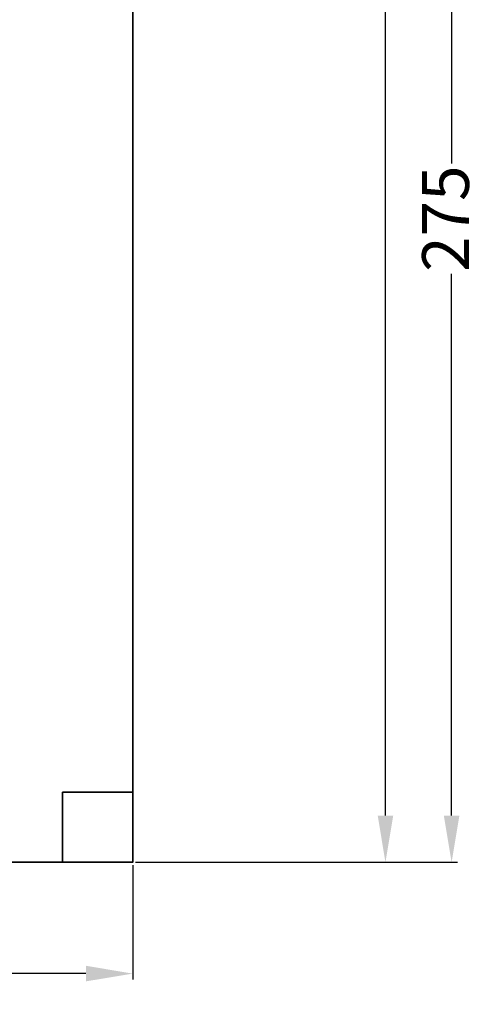
# Model space of a CAD drawing. Units: centimetres. Extents: x 2401 to 3632, y 2122 to 3526.
# Tile 4 of 10: x 3221 to 3320, y 2381 to 2591. Entities that reach past the tile are written whole.
import ezdxf

# ---------------------------------------------------------------- set-up
doc = ezdxf.new("R2010")
doc.units = ezdxf.units.CM
for name, color, linetype, lineweight in [('A-ANNO-DIMS', 9, 'Continuous', 18), ('A-COLS', 7, 'Continuous', 35), ('A-WALL', 7, 'Continuous', 35)]:
    doc.layers.add(name, color=color, linetype=linetype, lineweight=lineweight)
doc.styles.get("Standard").update_dxf_attribs({"font": 'arial.ttf'})
doc.dimstyles.new('ISO-25', dxfattribs={"dimtxt": 10, "dimasz": 10, "dimexe": 1.25, "dimexo": 0.625, "dimtad": 0, "dimtxsty": 'Standard', "dimcen": 2.5, "dimadec": 0, "dimazin": 0, "dimtfac": 1, "dimtmove": 0, "dimatfit": 3, "dimfxl": 1, "dimarcsym": 0})

# ---------------------------------------------------------------- blocks, each defined once
blk = doc.blocks.new('*D14')
at = {"layer": 'A-ANNO-DIMS', "color": 0, "lineweight": -2, "transparency": 16777216}
for p, q in [((3246.06, 3451.1), (3300.7, 3451.1)), ((3299.45, 3441.1), (3299.45, 2946.17)), ((3299.45, 2421.1), (3299.45, 2916.04)), ((3246.06, 2411.1), (3300.7, 2411.1))]:
    blk.add_line(p, q, dxfattribs=at)
at = {"layer": 'A-ANNO-DIMS', "color": 0, "transparency": 16777216}
for points in [[(3297.79, 3441.1), (3301.12, 3441.1), (3299.45, 3451.1)], [(3297.79, 2421.1), (3301.12, 2421.1), (3299.45, 2411.1)]]:
    blk.add_solid(points, dxfattribs=at)
at = {"layer": 'Defpoints', "color": 0, "transparency": 16777216}
for p in [(3245.44, 3451.1), (3245.44, 2411.1), (3299.45, 2411.1)]:
    blk.add_point(p, dxfattribs=at)
at = {"layer": 'A-ANNO-DIMS', "color": 0, "transparency": 16777216, "insert": (3299.45, 2931.1), "char_height": 10, "attachment_point": 5, "rotation": 90}
blk.add_mtext('1040', dxfattribs=at)
blk = doc.blocks.new('*D15')
at = {"layer": 'A-ANNO-DIMS', "color": 0, "lineweight": -2, "transparency": 16777216}
for p, q in [((2885.44, 2410.48), (2885.44, 2386.08)), ((3245.44, 2410.48), (3245.44, 2386.08)), ((2895.44, 2387.33), (3053.78, 2387.33)), ((3235.44, 2387.33), (3077.09, 2387.33))]:
    blk.add_line(p, q, dxfattribs=at)
at = {"layer": 'A-ANNO-DIMS', "color": 0, "transparency": 16777216}
for points in [[(2895.44, 2389), (2895.44, 2385.67), (2885.44, 2387.33)], [(3235.44, 2389), (3235.44, 2385.67), (3245.44, 2387.33)]]:
    blk.add_solid(points, dxfattribs=at)
at = {"layer": 'Defpoints', "color": 0, "transparency": 16777216}
for p in [(2885.44, 2411.1), (3245.44, 2411.1), (3245.44, 2387.33)]:
    blk.add_point(p, dxfattribs=at)
at = {"layer": 'A-ANNO-DIMS', "color": 0, "transparency": 16777216, "insert": (3065.44, 2387.33), "char_height": 10, "attachment_point": 5}
blk.add_mtext('360', dxfattribs=at)
blk = doc.blocks.new('*D43')
at = {"layer": 'A-ANNO-DIMS', "color": 0, "lineweight": -2, "transparency": 16777216}
for p, q in [((3246.06, 2686.1), (3314.84, 2686.1)), ((3313.59, 2676.1), (3313.59, 2560.4)), ((3313.59, 2421.1), (3313.59, 2536.81)), ((3246.06, 2411.1), (3314.84, 2411.1))]:
    blk.add_line(p, q, dxfattribs=at)
at = {"layer": 'A-ANNO-DIMS', "color": 0, "transparency": 16777216}
for points in [[(3311.92, 2676.1), (3315.25, 2676.1), (3313.59, 2686.1)], [(3311.92, 2421.1), (3315.25, 2421.1), (3313.59, 2411.1)]]:
    blk.add_solid(points, dxfattribs=at)
at = {"layer": 'Defpoints', "color": 0, "transparency": 16777216}
for p in [(3245.44, 2686.1), (3313.59, 2686.1), (3245.44, 2411.1)]:
    blk.add_point(p, dxfattribs=at)
at = {"layer": 'A-ANNO-DIMS', "color": 0, "transparency": 16777216, "insert": (3313.59, 2548.6), "char_height": 10, "attachment_point": 5, "rotation": 90}
blk.add_mtext('275', dxfattribs=at)

msp = doc.modelspace()

# ---------------------------------------------------------------- linework, layer by layer
at = {"layer": 'A-COLS'}
for p, q in [((3230.436, 2411.104), (3230.436, 2426.104)), ((3230.436, 2426.104), (3245.436, 2426.104)), ((3245.436, 2411.104), (3230.436, 2411.104))]:
    msp.add_line(p, q, dxfattribs=at)
at = {"layer": 'A-WALL'}
msp.add_lwpolyline([(2885.436, 2411.104), (3245.436, 2411.104), (3245.436, 3451.104), (2860.436, 3451.104)], dxfattribs=at)

# ---------------------------------------------------------------- dimensions: what is measured, and where the dimension line sits
at = {"layer": 'A-ANNO-DIMS'}
for base, p1, p2, override, picture, middle in [((3299.454, 2411.104), (3245.436, 3451.104), (3245.436, 2411.104), {"dimclrd": 0, "dimclre": 0, "dimclrt": 0}, '*D14', (3299.454, 2931.104)), ((3313.586, 2686.104), (3245.436, 2411.104), (3245.436, 2686.104), {"dimdec": 0, "dimlfac": 1, "dimrnd": 0, "dimzin": 0, "dimdsep": 46, "dimlunit": 2}, '*D43', (3313.586, 2548.604))]:
    dim = msp.add_linear_dim(base=base, p1=p1, p2=p2, angle=90, dimstyle='ISO-25', override=override, dxfattribs=at)
    dim.commit()
    dim.dimension.update_dxf_attribs({"geometry": picture, "text_midpoint": middle})
dim = msp.add_linear_dim(base=(3245.436, 2387.332), p1=(2885.436, 2411.104), p2=(3245.436, 2411.104), dimstyle='ISO-25', override={"dimclrd": 0, "dimclre": 0, "dimclrt": 0}, dxfattribs=at)
dim.commit()
dim.dimension.update_dxf_attribs({"geometry": '*D15', "text_midpoint": (3065.436, 2387.332)})

doc.saveas('drawing.dxf')
